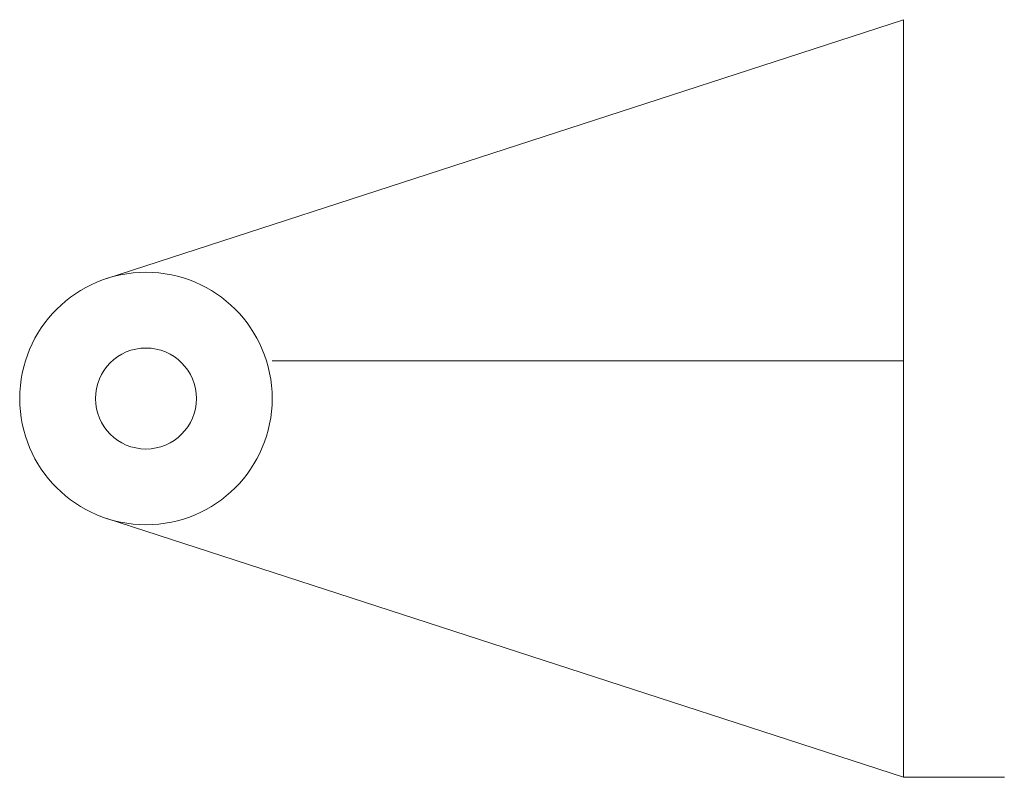
# Model space of a CAD drawing. Units: millimetres. Extents: x 3688 to 3844, y 1665 to 1785.
import ezdxf

# ---------------------------------------------------------------- set-up
doc = ezdxf.new("R2010")
doc.units = ezdxf.units.MM
doc.layers.add('M-CONS', color=8, linetype='Continuous', lineweight=18)

msp = doc.modelspace()

# ---------------------------------------------------------------- linework, layer by layer
at = {"layer": 'M-CONS'}
for p, q in [((3827.62, 1785.01), (3701.44, 1744.03)), ((3827.62, 1725.01), (3827.62, 1785.01)), ((3827.62, 1725.01), (3827.62, 1665.01)), ((3827.62, 1725.01, 16), (3827.62, 1725.01, 16)), ((3827.62, 1665.01), (3701.44, 1705.99))]:
    msp.add_line(p, q, dxfattribs=at)
at = {"layer": 'M-CONS', "extrusion": (0, -1, 0), "elevation": -1730.97}
msp.add_lwpolyline([(3757.62, 61), (3727.62, 16), (3827.62, 16), (3827.62, 81), (3777.62, 81)], dxfattribs=at)
at = {"layer": 'M-CONS', "extrusion": (0, -1, 0), "elevation": -1665.01}
msp.add_lwpolyline([(3843.62, 16), (3827.62, 16), (3827.62, 0), (3843.62, 0)], close=True, dxfattribs=at)
at = {"layer": 'M-CONS'}
for radius in [20, 8]:
    msp.add_circle((3707.62, 1725.01), radius, dxfattribs=at)
at = {"layer": 'M-CONS', "extrusion": (0, -1, 0)}
for radius in [20, 8]:
    msp.add_circle((3777.62, 61, -1730.97), radius, dxfattribs=at)

doc.saveas('drawing.dxf')
